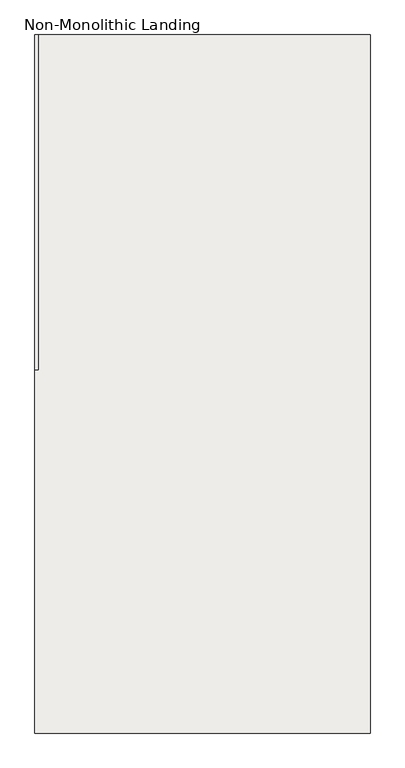
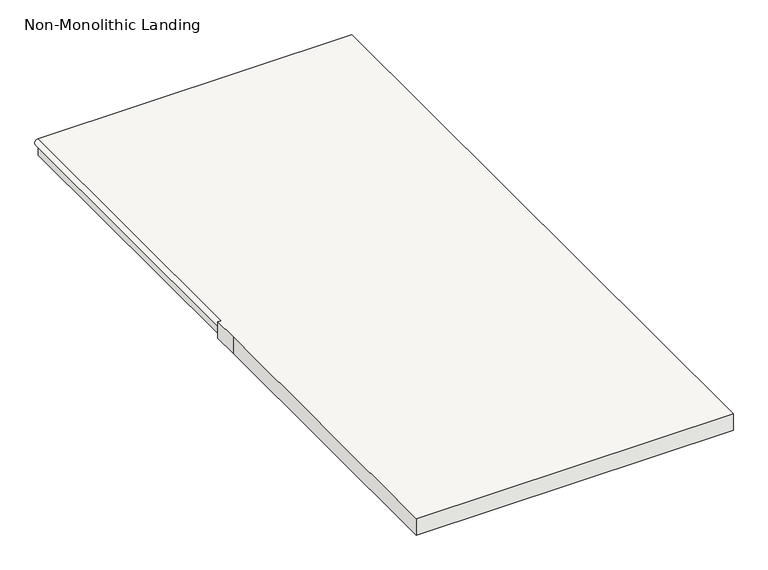
"""IFC4 building model written with IfcOpenShell, lengths in millimetres: slab geometry, Non-Monolithic Landing."""

from ifc_helpers import new_model, si_unit, frame, origin, place, context, project, spatial, circle_curve, source, transform, mapped, element, save
from ifc_brep_helpers import plane_surface, cylinder_surface, advanced_brep


def non_monolithic_landing_adbeca5e(model_context):
    return source(origin(), model_context, "Body", "AdvancedBrep", [
        advanced_brep(
        [(-7544.2282945, -3247.1921603, 1778.0), (-7554.2282945, -3247.1921603, 1778.0), (-7554.2282945, -3323.3921603, 1778.0), (-7554.2282945, -4237.7921603, 1778.0), (-6639.8282945, -4237.7921603, 1778.0), (-6639.8282945, -2332.7921603, 1778.0), (-7544.2282945, -2332.7921603, 1778.0), (-7544.2282945, -3247.1921603, 1728.0), (-7544.2282945, -2332.7921603, 1728.0), (-6639.8282945, -2332.7921603, 1728.0), (-6639.8282945, -4237.7921603, 1728.0), (-7554.2282945, -4237.7921603, 1728.0), (-7554.2282945, -3323.3921603, 1728.0), (-7554.2282945, -3247.1921603, 1728.0), (-7544.2282945, -3247.1921603, 1758.0), (-7544.2282945, -2332.7921603, 1758.0), (-7554.2282945, -3247.1921603, 1768.0)],
        [
            (0, 1),
            (1, 2),
            (2, 3),
            (3, 4),
            (4, 5),
            (5, 6),
            (6, 0),
            (7, 8),
            (8, 9),
            (9, 10),
            (10, 11),
            (11, 12),
            (12, 13),
            (13, 7),
            (7, 14),
            (14, 15),
            (15, 8),
            (1, 16),
            (16, 13),
            (12, 2),
            (11, 3),
            (10, 4),
            (9, 5),
            (15, 6, circle_curve(frame((-7544.2282945, -2332.7921603, 1768.0), z_axis=(0.0, 1.0, 0.0), x_axis=(1.0, 0.0, 0.0)), 10.0)),
            (14, 16, circle_curve(frame((-7544.2282945, -3247.1921603, 1768.0), z_axis=(0.0, 1.0, 0.0), x_axis=(1.0, 0.0, 0.0)), 10.0)),
            (16, 0, circle_curve(frame((-7544.2282945, -3247.1921603, 1768.0), z_axis=(0.0, 1.0, 0.0), x_axis=(1.0, 0.0, 0.0)), 10.0)),
        ],
        [
            plane_surface(frame((-7544.2282945, -2332.7921603, 1778.0), z_axis=(0.0, 0.0, 1.0), x_axis=(0.0, -1.0, 0.0))),
            plane_surface(frame((-7544.2282945, -2332.7921603, 1728.0), z_axis=(0.0, 0.0, -1.0), x_axis=(0.0, 1.0, 0.0))),
            plane_surface(frame((-7544.2282945, -2332.7921603, 1778.0), z_axis=(-1.0, 0.0, 0.0), x_axis=(0.0, 0.0, -1.0))),
            plane_surface(frame((-7554.2282945, -3247.1921603, 1778.0), z_axis=(-1.0, 0.0, 0.0), x_axis=(0.0, 0.0, -1.0))),
            plane_surface(frame((-7554.2282945, -3323.3921603, 1778.0), z_axis=(-1.0, 0.0, 0.0), x_axis=(0.0, 0.0, -1.0))),
            plane_surface(frame((-7554.2282945, -4237.7921603, 1778.0), z_axis=(0.0, -1.0, 0.0), x_axis=(0.0, 0.0, -1.0))),
            plane_surface(frame((-6639.8282945, -4237.7921603, 1778.0), z_axis=(1.0, 0.0, 0.0), x_axis=(0.0, 0.0, -1.0))),
            plane_surface(frame((-6639.8282945, -2332.7921603, 1778.0), z_axis=(0.0, 1.0, 0.0), x_axis=(0.0, 0.0, -1.0))),
            cylinder_surface(frame((-7544.2282945, -3247.1921603, 1768.0), z_axis=(0.0, -1.0, 0.0), x_axis=(1.0, 0.0, 0.0)), 10.0),
            plane_surface(frame((-7544.2282945, -3247.1921603, 1778.0), z_axis=(0.0, 1.0, 0.0), x_axis=(0.0, 0.0, -1.0))),
        ],
        [
            (0, [[1, 2, 3, 4, 5, 6, 7]]),
            (1, [[8, 9, 10, 11, 12, 13, 14]]),
            (2, [[-8, 15, 16, 17]]),
            (3, [[-2, 18, 19, -13, 20]]),
            (4, [[-3, -20, -12, 21]]),
            (5, [[-4, -21, -11, 22]]),
            (6, [[-5, -22, -10, 23]]),
            (7, [[-6, -23, -9, -17, 24]]),
            (8, [[-24, -16, 25, 26, -7]]),
            (9, [[-1, -26, -18]]),
            (9, [[-14, -19, -25, -15]]),
        ],
    ),
    ])


if __name__ == "__main__":
    model = new_model("IFC4")
    model_context = context("Model", 3, world=origin())
    ifc_project = project(units=[si_unit("LENGTHUNIT", "METRE", prefix="MILLI")], contexts=[model_context])
    site = spatial("IfcSite", under=ifc_project)
    building = spatial("IfcBuilding", under=site)
    placement = place(None, origin())
    non_monolithic_landing_shape = non_monolithic_landing_adbeca5e(model_context)
    element("IfcSlab", 1, ObjectType="Non-Monolithic Landing", at=placement, inside=building, context=model_context, shape_type="MappedRepresentation", body=[
        mapped(non_monolithic_landing_shape, transform((0.0, 0.0, 0.0), x_axis=(1.0, 0.0, 0.0), y_axis=(0.0, 1.0, 0.0), z_axis=(0.0, 0.0, 1.0))),
    ])
    save(model, "model.ifc")
